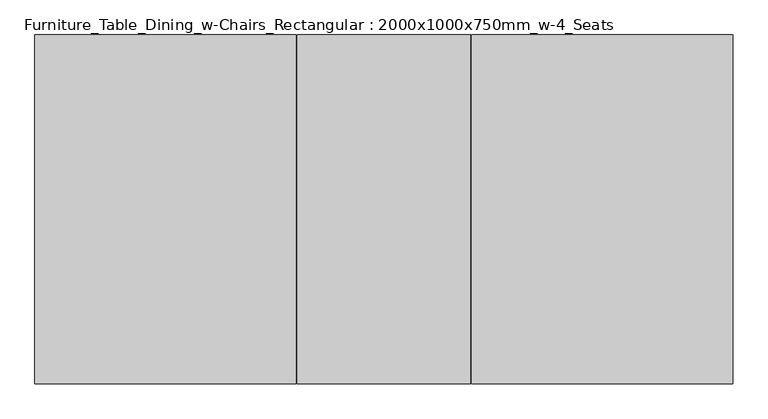
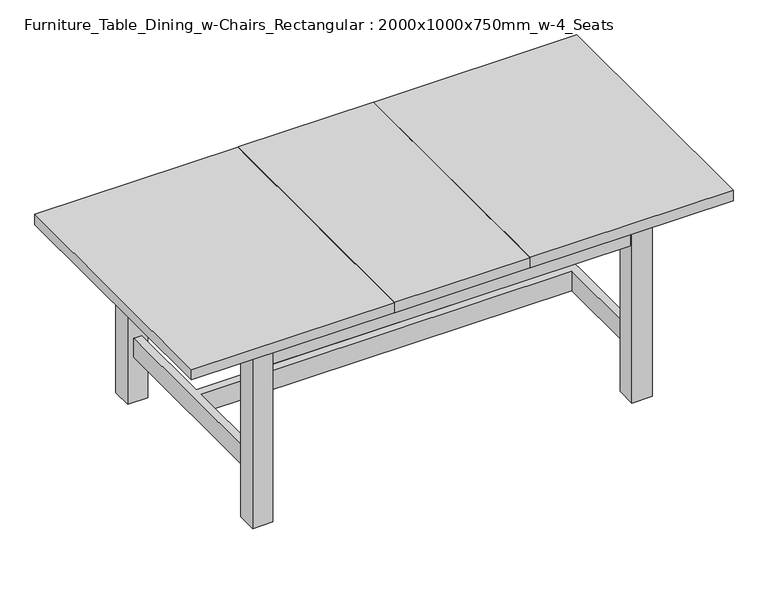
"""IFC4 building model written with IfcOpenShell, lengths in millimetres: furniture geometry, Furniture_Table_Dining_w-Chairs_Rectangular : 2000x1000x750mm_w-4_Seats."""

from ifc_helpers import new_model, si_unit, frame, origin, origin_with_axes, place, context, project, spatial, polyline, outline, extrude, faceted_brep, source, transform, mapped, element, save


def furniture_table_dining_w_chairs_rectangular_2000x1000x750mm_b8cbee69(model_context):
    return source(origin(), model_context, "Body", "SolidModel", [
        faceted_brep([(1118.1787219, -455.6453708, 750.0), (1118.1787219, 544.3546292, 750.0), (369.6787219, 544.3546292, 750.0), (369.6787219, -455.6453708, 750.0), (-881.8212781, 544.3546292, 750.0), (-881.8212781, -455.6453708, 750.0), (-133.3212781, -455.6453708, 750.0), (-133.3212781, 544.3546292, 750.0), (366.6787219, 544.3546292, 750.0), (-130.3212781, 544.3546292, 750.0), (-130.3212781, -455.6453708, 750.0), (366.6787219, -455.6453708, 750.0), (-881.8212781, -455.6453708, 710.0), (-881.8212781, 544.3546292, 710.0), (-133.3212781, 544.3546292, 710.0), (-131.8212781, 542.8546292, 710.0), (-130.3212781, 544.3546292, 710.0), (366.6787219, 544.3546292, 710.0), (368.1787219, 542.8546292, 710.0), (369.6787219, 544.3546292, 710.0), (1118.1787219, 544.3546292, 710.0), (1118.1787219, -455.6453708, 710.0), (369.6787219, -455.6453708, 710.0), (368.1787219, -454.1453708, 710.0), (366.6787219, -455.6453708, 710.0), (-130.3212781, -455.6453708, 710.0), (-131.8212781, -454.1453708, 710.0), (-133.3212781, -455.6453708, 710.0), (-131.8212781, 542.8546292, 748.5), (368.1787219, 542.8546292, 748.5), (-131.8212781, -454.1453708, 748.5), (368.1787219, -454.1453708, 748.5)], [[[0, 1, 2, 3]], [[4, 5, 6, 7]], [[8, 9, 10, 11]], [[12, 13, 14, 15, 16, 17, 18, 19, 20, 21, 22, 23, 24, 25, 26, 27]], [[1, 0, 21, 20]], [[9, 8, 17, 16]], [[1, 20, 19, 2]], [[13, 4, 7, 14]], [[5, 4, 13, 12]], [[11, 10, 25, 24]], [[21, 0, 3, 22]], [[5, 12, 27, 6]], [[15, 28, 9, 16]], [[28, 15, 14, 7]], [[18, 29, 2, 19]], [[29, 18, 17, 8]], [[9, 28, 30, 10]], [[28, 7, 6, 30]], [[2, 29, 31, 3]], [[29, 8, 11, 31]], [[10, 30, 26, 25]], [[30, 6, 27, 26]], [[3, 31, 23, 22]], [[31, 11, 24, 23]]]),
        extrude(outline(polyline([(-544.3212781, -393.1453708), (-619.3212781, -393.1453708), (-619.3212781, -318.1453708), (-544.3212781, -318.1453708), (-544.3212781, -393.1453708)])), origin_with_axes(), (0.0, 0.0, 1.0), 710.0),
        extrude(outline(polyline([(780.6787219, 481.8546292), (855.6787219, 481.8546292), (855.6787219, 406.8546292), (780.6787219, 406.8546292), (780.6787219, 481.8546292)])), origin_with_axes(), (0.0, 0.0, 1.0), 710.0),
        extrude(outline(polyline([(780.6787219, -318.1453708), (855.6787219, -318.1453708), (855.6787219, -393.1453708), (780.6787219, -393.1453708), (780.6787219, -318.1453708)])), origin_with_axes(), (0.0, 0.0, 1.0), 710.0),
        extrude(outline(polyline([(-544.3212781, 481.8546292), (-544.3212781, 406.8546292), (-619.3212781, 406.8546292), (-619.3212781, 481.8546292), (-544.3212781, 481.8546292)])), origin_with_axes(), (0.0, 0.0, 1.0), 710.0),
        extrude(outline(polyline([(-566.8212781, -318.1453708), (-596.8212781, -318.1453708), (-596.8212781, 406.8546292), (-566.8212781, 406.8546292), (-566.8212781, 59.3546292), (803.1787219, 59.3546292), (803.1787219, 406.8546292), (833.1787219, 406.8546292), (833.1787219, -318.1453708), (803.1787219, -318.1453708), (803.1787219, 29.3546292), (-566.8212781, 29.3546292), (-566.8212781, -318.1453708)])), frame((0.0, 0.0, 175.0), z_axis=(0.0, 0.0, 1.0), x_axis=(1.0, 0.0, 0.0)), (0.0, 0.0, 1.0), 75.0),
        extrude(outline(polyline([(-544.3212781, 474.3546292), (780.6787219, 474.3546292), (780.6787219, 454.3546292), (-544.3212781, 454.3546292), (-544.3212781, 474.3546292)])), frame((0.0, 0.0, 610.0), z_axis=(0.0, 0.0, 1.0), x_axis=(1.0, 0.0, 0.0)), (0.0, 0.0, 1.0), 100.0),
        extrude(outline(polyline([(-611.8212781, -318.1453708), (-611.8212781, 406.8546292), (-591.8212781, 406.8546292), (-591.8212781, -318.1453708), (-611.8212781, -318.1453708)])), frame((0.0, 0.0, 610.0), z_axis=(0.0, 0.0, 1.0), x_axis=(1.0, 0.0, 0.0)), (0.0, 0.0, 1.0), 100.0),
        extrude(outline(polyline([(780.6787219, -385.6453708), (-544.3212781, -385.6453708), (-544.3212781, -365.6453708), (780.6787219, -365.6453708), (780.6787219, -385.6453708)])), frame((0.0, 0.0, 610.0), z_axis=(0.0, 0.0, 1.0), x_axis=(1.0, 0.0, 0.0)), (0.0, 0.0, 1.0), 100.0),
        extrude(outline(polyline([(848.1787219, 406.8546292), (848.1787219, -318.1453708), (828.1787219, -318.1453708), (828.1787219, 406.8546292), (848.1787219, 406.8546292)])), frame((0.0, 0.0, 610.0), z_axis=(0.0, 0.0, 1.0), x_axis=(1.0, 0.0, 0.0)), (0.0, 0.0, 1.0), 100.0),
    ])


if __name__ == "__main__":
    model = new_model("IFC4")
    model_context = context("Model", 3, world=origin())
    ifc_project = project(units=[si_unit("LENGTHUNIT", "METRE", prefix="MILLI")], contexts=[model_context])
    site = spatial("IfcSite", under=ifc_project)
    building = spatial("IfcBuilding", under=site)
    placement = place(None, origin())
    furniture_table_dining_w_chairs_rectangular_2000x1000x750mm_shape = furniture_table_dining_w_chairs_rectangular_2000x1000x750mm_b8cbee69(model_context)
    element("IfcFurniture", 1, ObjectType="Furniture_Table_Dining_w-Chairs_Rectangular : 2000x1000x750mm_w-4_Seats", at=placement, inside=building, context=model_context, shape_type="MappedRepresentation", body=[
        mapped(furniture_table_dining_w_chairs_rectangular_2000x1000x750mm_shape, transform((0.0, 0.0, 0.0), x_axis=(1.0, 0.0, 0.0), y_axis=(0.0, 1.0, 0.0), z_axis=(0.0, 0.0, 1.0))),
    ])
    save(model, "model.ifc")

# Revit data of these elements
# Type "Furniture_Table_Dining_w-Chairs_Rectangular : 2000x1000x750mm_w-4_Seats"
#   Keynote = "N"
#   Width = 3' - 3.37008"
#   Table Top Thickness = 0' - 1.5748"
#   Table Height = 2' - 5.52756"
#   Length = 6' - 6.74016"
#   Leg Width = 0' - 2.95276"
#   Leg Spacing Width = 2' - 7.49606"
#   Leg Spacing Length = 4' - 7.11811"
#   Chair Side Spacing = 2' - 3.55906"
#   Centre Piece = 1' - 7.68504"
#   Vis - End Chairs = no
#   Material Table = Wood - Birch
#   Material Chair Structure = Wood - Birch
#   Material Chair Covering = Fabric - Beige
#   Default Elevation = 0
# Element 1 (IfcFurniture, "Furniture_Table_Dining_w-Chairs_Rectangular : 2000x1000x750mm_w-4_Seats")
#   Materials on its faces: "Wood - Birch"
# Materials
#   "Wood - Birch": class "Wood", colour RGB 224 178 126, transparency 0
#   "Fabric - Beige": class "Fabric", colour RGB 231 227 195, transparency 0
